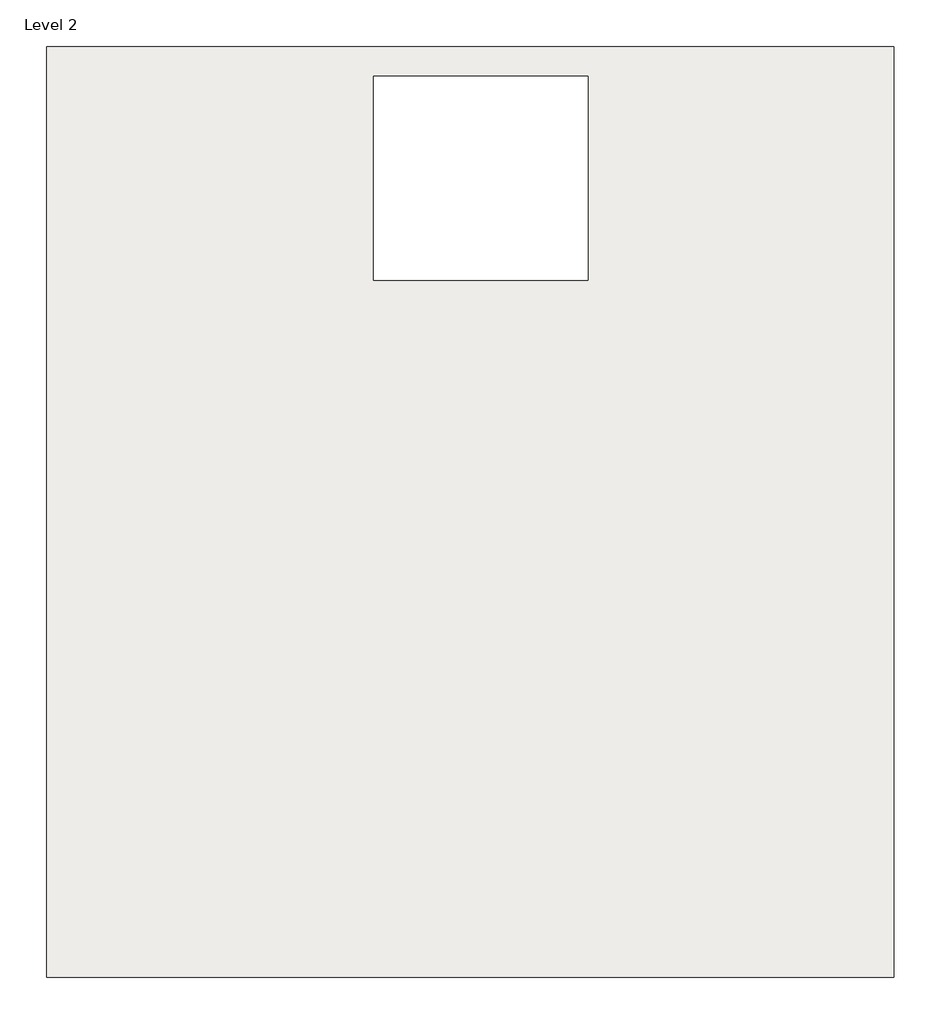
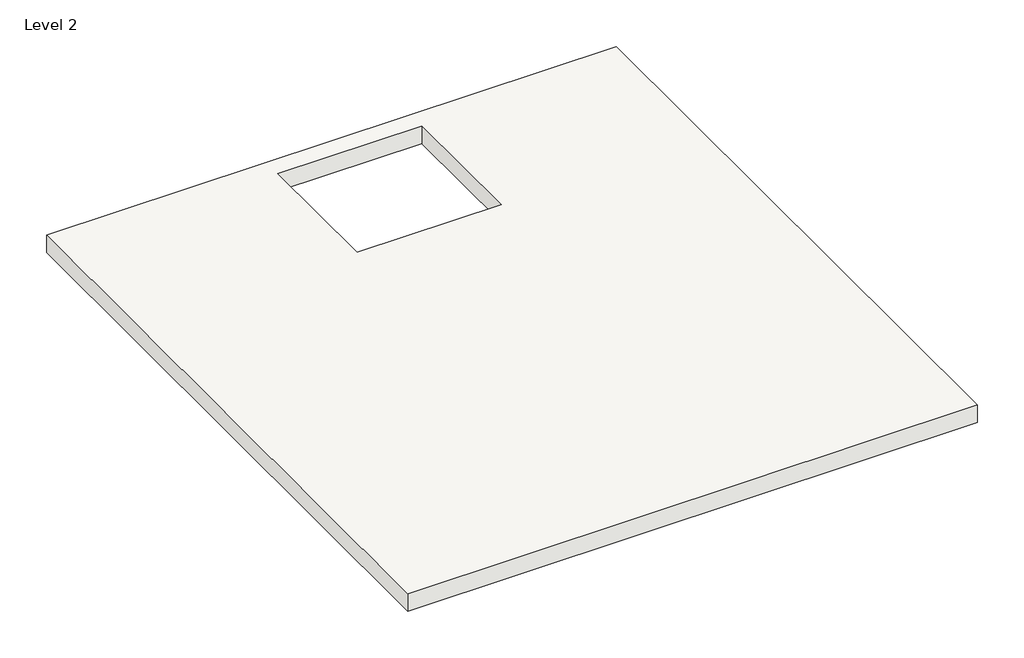
# One storey: 1 roof.
"""IFC4 building model written with IfcOpenShell, lengths in millimetres."""

from ifc_helpers import new_model, si_unit, frame, origin, place, context, project, spatial, polyline, outline, extrude, element, save

model = new_model("IFC4")

# Units and contexts
model_context = context("Model", 3, world=origin())
ifc_project = project(units=[si_unit("LENGTHUNIT", "METRE", prefix="MILLI")], contexts=[model_context])

# Site, building, storey
site = spatial("IfcSite", under=ifc_project)
building = spatial("IfcBuilding", under=site)
storey = spatial("IfcBuildingStorey", under=building, Name="Level 2", Elevation=3048.0)

# Roof
placement = place(None, origin())
element("IfcRoof", 1, ObjectType="Generic - 12\"", at=placement, inside=storey, context=model_context, shape_type="SweptSolid", body=[
    extrude(outline(polyline([(-11898.0611447, 11435.685558), (-2550.8611447, 11435.685558), (-2550.8611447, 1174.085558), (-11898.0611447, 1174.085558), (-11898.0611447, 11435.685558)]), holes=[polyline([(-8291.2611447, 11109.2172498), (-8291.2611447, 8859.8360051), (-5929.0611447, 8859.8360051), (-5929.0611447, 11109.2172498), (-8291.2611447, 11109.2172498)])]), frame((0.0, 0.0, 3048.0), z_axis=(0.0, 0.0, 1.0), x_axis=(1.0, 0.0, 0.0)), (0.0, 0.0, 1.0), 304.8),
])

save(model, "model.ifc")

# Revit data of these elements
# Type "Generic - 12\""
#   Assembly Code = "B1020"
#   Layers, outside or top first: 1' - 0" no material (function 1)
# Element 1 (IfcRoof, "Generic - 12\"")
#   built-in parameter 1001705 = 11 (stored number, unit not read)
#   built-in parameter 1001710 = 33615
#   Phase Created = New Construction
#   Materials on its faces: "Default Roof"
# Materials
#   "Default Roof": colour RGB 88 101 114, transparency 0
